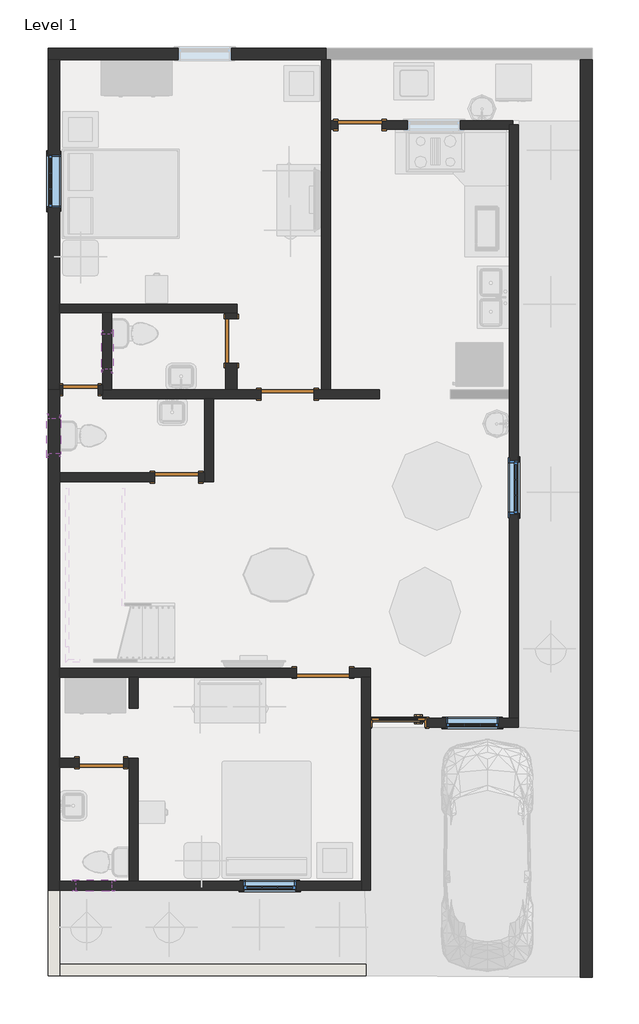
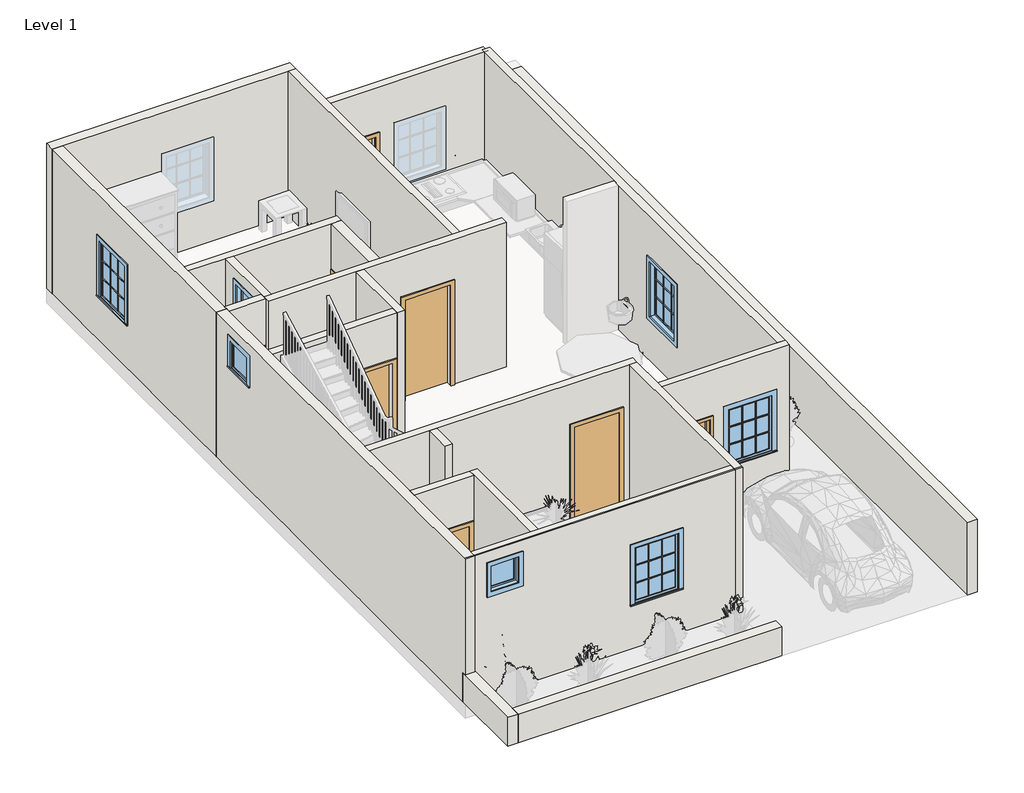
# One storey, part 1 of 3: 23 walls, 8 doors, 7 windows.
"""IFC4 building model written with IfcOpenShell, lengths in millimetres."""

from ifc_helpers import new_model, si_unit, frame, origin, origin_with_axes, place, context, project, spatial, polyline, outline, extrude, faceted_brep, transform, mapped, element, save
from components import door_808aeb8e, door_d7591924, door_fadea3f2, door_255cab33, door_059fdd7e, door_16372e1c, door_686f89d2, window_29c06734, window_5c190c7e, window_3d781103, window_e41d21a6

model = new_model("IFC4")

# Units and contexts
model_context = context("Model", 3, world=origin())
ifc_project = project(units=[si_unit("LENGTHUNIT", "METRE", prefix="MILLI")], contexts=[model_context])

# Site, building, storey
site = spatial("IfcSite", under=ifc_project)
building = spatial("IfcBuilding", under=site)
storey = spatial("IfcBuildingStorey", under=building, Name="Level 1", Elevation=0.0)

# Doors
placement = place(None, origin())
door_shape = door_808aeb8e(model_context)
element("IfcDoor", 1, ObjectType="36\" x 80\"", at=placement, inside=storey, context=model_context, shape_type="MappedRepresentation", body=[
    mapped(door_shape, transform((-8513.5660538, 2790.728629, 0.0), x_axis=(1.0, 0.0, 0.0), y_axis=(0.0, 1.0, 0.0), z_axis=(0.0, 0.0, 1.0))),
])
door_2_shape = door_d7591924(model_context)
element("IfcDoor", 2, ObjectType="Single-Flush : 24\" x 80\"", at=placement, inside=storey, context=model_context, shape_type="MappedRepresentation", body=[
    mapped(door_2_shape, transform((-13974.5660538, 8502.553629, 0.0), x_axis=(1.0, 0.0, 0.0), y_axis=(0.0, 1.0, 0.0), z_axis=(0.0, 0.0, 1.0))),
])
door_3_shape = door_fadea3f2(model_context)
element("IfcDoor", 3, ObjectType="Single-Flush : 30\" x 80\"", at=placement, inside=storey, context=model_context, shape_type="MappedRepresentation", body=[
    mapped(door_3_shape, transform((-11383.7660538, 9340.753629, 0.0), x_axis=(0.0, 1.0, 0.0), y_axis=(-1.0, 0.0, 0.0), z_axis=(0.0, 0.0, 1.0))),
])
door_4_shape = door_255cab33(model_context)
element("IfcDoor", 4, ObjectType="Single-Flush : 30\" x 80\"", at=placement, inside=storey, context=model_context, shape_type="MappedRepresentation", body=[
    mapped(door_4_shape, transform((-9173.9660538, 13049.153629, 0.0), x_axis=(-1.0, 0.0, 0.0), y_axis=(0.0, -1.0, 0.0), z_axis=(0.0, 0.0, 1.0))),
])
element("IfcDoor", 5, ObjectType="Single-Flush : 30\" x 80\"", at=placement, inside=storey, context=model_context, shape_type="MappedRepresentation", body=[
    mapped(door_4_shape, transform((-13618.9660538, 2101.753629, 0.0), x_axis=(1.0, 0.0, 0.0), y_axis=(0.0, 1.0, 0.0), z_axis=(0.0, 0.0, 1.0))),
])
door_5_shape = door_059fdd7e(model_context)
element("IfcDoor", 6, ObjectType="Single-Flush : 30\" x 80\"", at=placement, inside=storey, context=model_context, shape_type="MappedRepresentation", body=[
    mapped(door_5_shape, transform((-12323.5660538, 7003.953629, 0.0), x_axis=(1.0, 0.0, 0.0), y_axis=(0.0, 1.0, 0.0), z_axis=(0.0, 0.0, 1.0))),
])
door_6_shape = door_16372e1c(model_context)
element("IfcDoor", 7, ObjectType="Single-Flush : 36\" x 84\"", at=placement, inside=storey, context=model_context, shape_type="MappedRepresentation", body=[
    mapped(door_6_shape, transform((-10418.5660538, 8426.353629, 0.0), x_axis=(1.0, 0.0, 0.0), y_axis=(0.0, 1.0, 0.0), z_axis=(0.0, 0.0, 1.0))),
])
door_7_shape = door_686f89d2(model_context)
element("IfcDoor", 8, ObjectType="Single-Flush : 36\" x 84\"", at=placement, inside=storey, context=model_context, shape_type="MappedRepresentation", body=[
    mapped(door_7_shape, transform((-9808.9660538, 3651.153629, 0.0), x_axis=(1.0, 0.0, 0.0), y_axis=(0.0, 1.0, 0.0), z_axis=(0.0, 0.0, 1.0))),
])

# Walls
element("IfcWall", 9, ObjectType="Generic - 8\"", at=placement, inside=storey, context=model_context, shape_type="Brep", body=[
    faceted_brep([(-14533.3660538, 14166.753629, 0.0), (-14330.1660538, 14166.753629, 0.0), (-9834.3660538, 14166.753629, 0.0), (-9758.1660538, 14166.753629, 0.0), (-9758.1660538, 14166.753629, 1524.0), (-9681.9660538, 14166.753629, 1524.0), (-9681.9660538, 14166.753629, 3048.0), (-9834.3660538, 14166.753629, 3048.0), (-14330.1660538, 14166.753629, 3048.0), (-14533.3660538, 14166.753629, 3048.0), (-11383.7660538, 14166.753629, 2133.6), (-11383.7660538, 14166.753629, 914.4), (-12298.1660538, 14166.753629, 914.4), (-12298.1660538, 14166.753629, 2133.6), (-14533.3660538, 14369.953629, 0.0), (-14533.3660538, 14369.953629, 3048.0), (-9681.9660538, 14369.953629, 3048.0), (-9681.9660538, 14369.953629, 1524.0), (-9758.1660538, 14369.953629, 1524.0), (-9758.1660538, 14369.953629, 0.0), (-11383.7660538, 14369.953629, 2133.6), (-12298.1660538, 14369.953629, 2133.6), (-12298.1660538, 14369.953629, 914.4), (-11383.7660538, 14369.953629, 914.4)], [[[0, 1, 2, 3, 4, 5, 6, 7, 8, 9], [10, 11, 12, 13]], [[14, 15, 16, 17, 18, 19], [20, 21, 22, 23]], [[3, 2, 1, 0, 14, 19]], [[0, 9, 15, 14]], [[11, 10, 20, 23]], [[12, 11, 23, 22]], [[13, 12, 22, 21]], [[10, 13, 21, 20]], [[4, 3, 19, 18]], [[17, 5, 4, 18]], [[6, 5, 17, 16]], [[9, 8, 7, 6, 16, 15]]]),
])
element("IfcWall", 10, ObjectType="Generic - 8\"", at=placement, inside=storey, context=model_context, shape_type="SweptSolid", body=[
    extrude(outline(polyline([(9823.353629, 0.0), (9721.753629, 0.0), (9721.753629, 2032.0), (8959.753629, 2032.0), (8959.753629, 0.0), (8502.553629, 0.0), (8502.553629, 3048.0), (9823.353629, 3048.0), (9823.353629, 0.0)])), frame((-11485.3660538, 0.0, 0.0), z_axis=(1.0, 0.0, 0.0), x_axis=(0.0, 1.0, 0.0)), (0.0, 0.0, 1.0), 203.2),
])
element("IfcWall", 11, ObjectType="Generic - 8\"", at=placement, inside=storey, context=model_context, shape_type="Brep", body=[
    faceted_brep([(-14330.1660538, 8502.553629, 0.0), (-14330.1660538, 8578.753629, 0.0), (-14330.1660538, 9823.353629, 0.0), (-14330.1660538, 9975.753629, 0.0), (-14330.1660538, 14166.753629, 0.0), (-14330.1660538, 14166.753629, 3048.0), (-14330.1660538, 9975.753629, 3048.0), (-14330.1660538, 9823.353629, 3048.0), (-14330.1660538, 8578.753629, 3048.0), (-14330.1660538, 8502.553629, 3048.0), (-14330.1660538, 12541.153629, 2133.6), (-14330.1660538, 12541.153629, 914.4), (-14330.1660538, 11626.753629, 914.4), (-14330.1660538, 11626.753629, 2133.6), (-14533.3660538, 8502.553629, 0.0), (-14533.3660538, 8502.553629, 3048.0), (-14533.3660538, 14166.753629, 3048.0), (-14533.3660538, 14166.753629, 0.0), (-14533.3660538, 12541.153629, 2133.6), (-14533.3660538, 11626.753629, 2133.6), (-14533.3660538, 11626.753629, 914.4), (-14533.3660538, 12541.153629, 914.4)], [[[0, 1, 2, 3, 4, 5, 6, 7, 8, 9], [10, 11, 12, 13]], [[14, 15, 16, 17], [18, 19, 20, 21]], [[4, 3, 2, 1, 0, 14, 17]], [[0, 9, 15, 14]], [[5, 4, 17, 16]], [[11, 10, 18, 21]], [[12, 11, 21, 20]], [[13, 12, 20, 19]], [[10, 13, 19, 18]], [[9, 8, 7, 6, 5, 16, 15]]]),
])
element("IfcWall", 12, ObjectType="Generic - 8\"", at=placement, inside=storey, context=model_context, shape_type="Brep", body=[
    faceted_brep([(-14330.1660538, -6.446371, 0.0), (-14330.1660538, 69.753629, 0.0), (-14330.1660538, 2025.553629, 0.0), (-14330.1660538, 2177.953629, 0.0), (-14330.1660538, 3574.953629, 0.0), (-14330.1660538, 3727.353629, 0.0), (-14330.1660538, 6927.753629, 0.0), (-14330.1660538, 7080.153629, 0.0), (-14330.1660538, 8426.353629, 0.0), (-14330.1660538, 8502.553629, 0.0), (-14330.1660538, 8502.553629, 3048.0), (-14330.1660538, 8426.353629, 3048.0), (-14330.1660538, 7080.153629, 3048.0), (-14330.1660538, 6927.753629, 3048.0), (-14330.1660538, 3727.353629, 3048.0), (-14330.1660538, 3574.953629, 3048.0), (-14330.1660538, 2177.953629, 3048.0), (-14330.1660538, 2025.553629, 3048.0), (-14330.1660538, 69.753629, 3048.0), (-14330.1660538, -50.896371, 3048.0), (-14330.1660538, -82.646371, 3048.0), (-14330.1660538, -82.646371, 609.6), (-14330.1660538, -6.446371, 609.6), (-14330.1660538, 8019.953629, 2768.6), (-14330.1660538, 8019.953629, 2159.0), (-14330.1660538, 7410.353629, 2159.0), (-14330.1660538, 7410.353629, 2768.6), (-14533.3660538, -6.446371, 0.0), (-14533.3660538, -6.446371, 609.6), (-14533.3660538, -82.646371, 609.6), (-14533.3660538, -82.646371, 3048.0), (-14533.3660538, -50.896371, 3048.0), (-14533.3660538, 8502.553629, 3048.0), (-14533.3660538, 8502.553629, 0.0), (-14533.3660538, 8019.953629, 2768.6), (-14533.3660538, 7410.353629, 2768.6), (-14533.3660538, 7410.353629, 2159.0), (-14533.3660538, 8019.953629, 2159.0)], [[[0, 1, 2, 3, 4, 5, 6, 7, 8, 9, 10, 11, 12, 13, 14, 15, 16, 17, 18, 19, 20, 21, 22], [23, 24, 25, 26]], [[27, 28, 29, 30, 31, 32, 33], [34, 35, 36, 37]], [[9, 8, 7, 6, 5, 4, 3, 2, 1, 0, 27, 33]], [[10, 9, 33, 32]], [[0, 22, 28, 27]], [[21, 29, 28, 22]], [[21, 20, 30, 29]], [[24, 23, 34, 37]], [[25, 24, 37, 36]], [[26, 25, 36, 35]], [[23, 26, 35, 34]], [[20, 19, 31, 30]], [[19, 18, 17, 16, 15, 14, 13, 12, 11, 10, 32, 31]]]),
])
element("IfcWall", 13, ObjectType="Generic - 8\" 2", at=placement, inside=storey, context=model_context, shape_type="SweptSolid", body=[
    extrude(outline(polyline([(-5389.3660538, -1581.246371), (-5389.3660538, 14166.753629), (-5186.1660538, 14166.753629), (-5186.1660538, -1581.246371), (-5389.3660538, -1581.246371)])), origin_with_axes(), (0.0, 0.0, 1.0), 1524.0),
])
element("IfcWall", 14, ObjectType="Generic - 8\" 2", at=placement, inside=storey, context=model_context, shape_type="Brep", body=[
    faceted_brep([(-14330.1660538, -1555.846371, 0.0), (-14330.1660538, -1352.646371, 0.0), (-14330.1660538, -82.646371, 0.0), (-14330.1660538, -6.446371, 0.0), (-14330.1660538, -6.446371, 609.6), (-14330.1660538, -1352.646371, 609.6), (-14330.1660538, -1555.846371, 609.6), (-14533.3660538, -1555.846371, 0.0), (-14533.3660538, -1555.846371, 609.6), (-14533.3660538, -6.446371, 609.6), (-14533.3660538, -6.446371, 0.0)], [[[0, 1, 2, 3, 4, 5, 6]], [[7, 8, 9, 10]], [[3, 2, 1, 0, 7, 10]], [[4, 3, 10, 9]], [[6, 5, 4, 9, 8]], [[0, 6, 8, 7]]]),
])
element("IfcWall", 15, ObjectType="Generic - 8\" 2", at=placement, inside=storey, context=model_context, shape_type="SweptSolid", body=[
    extrude(outline(polyline([(-14330.1660538, -1352.646371), (-9072.3660538, -1352.646371), (-9072.3660538, -1555.846371), (-14330.1660538, -1555.846371), (-14330.1660538, -1352.646371)])), origin_with_axes(), (0.0, 0.0, 1.0), 609.6),
])
element("IfcWall", 16, ObjectType="INNER 6\"", at=placement, inside=storey, context=model_context, shape_type="Brep", body=[
    faceted_brep([(-9834.3660538, 14166.753629, 3048.0), (-9834.3660538, 14166.753629, 0.0), (-9834.3660538, 8502.553629, 0.0), (-9834.3660538, 8502.553629, 3048.0), (-9681.9660538, 14166.753629, 0.0), (-9681.9660538, 14166.753629, 1524.0), (-9681.9660538, 14166.753629, 3048.0), (-9681.9660538, 13125.353629, 3048.0), (-9681.9660538, 12972.953629, 3048.0), (-9681.9660538, 8502.553629, 3048.0), (-9681.9660538, 8502.553629, 0.0), (-9681.9660538, 12972.953629, 0.0), (-9681.9660538, 13125.353629, 0.0), (-9758.1660538, 14166.753629, 0.0)], [[[0, 1, 2, 3]], [[4, 5, 6, 7, 8, 9, 10, 11, 12]], [[2, 1, 13, 4, 12, 11, 10]], [[3, 2, 10, 9]], [[0, 6, 5, 4, 13, 1]], [[0, 3, 9, 8, 7, 6]]]),
])
element("IfcWall", 17, ObjectType="INNER 6\"", at=placement, inside=storey, context=model_context, shape_type="SweptSolid", body=[
    extrude(outline(polyline([(0.0, -9681.9660538), (0.0, -9554.9660538), (2032.0, -9554.9660538), (2032.0, -8792.9660538), (0.0, -8792.9660538), (0.0, -6545.0660538), (3048.0, -6545.0660538), (3048.0, -9681.9660538), (0.0, -9681.9660538)]), holes=[polyline([(2133.6, -7446.7660538), (914.4, -7446.7660538), (914.4, -8361.1660538), (2133.6, -8361.1660538), (2133.6, -7446.7660538)])]), frame((0.0, 12972.953629, 0.0), z_axis=(0.0, 1.0, 0.0), x_axis=(0.0, 0.0, 1.0)), (0.0, 0.0, 1.0), 152.4),
])
element("IfcWall", 18, ObjectType="INNER 6\"", at=placement, inside=storey, context=model_context, shape_type="Brep", body=[
    faceted_brep([(-6456.1660538, 2863.753629, 0.0), (-6456.1660538, 13049.153629, 0.0), (-6456.1660538, 13049.153629, 3048.0), (-6456.1660538, 2863.753629, 3048.0), (-6456.1660538, 6368.953629, 2133.6), (-6456.1660538, 7283.353629, 2133.6), (-6456.1660538, 7283.353629, 914.4), (-6456.1660538, 6368.953629, 914.4), (-6608.5660538, 2863.753629, 0.0), (-6608.5660538, 2863.753629, 3048.0), (-6608.5660538, 8350.153629, 3048.0), (-6608.5660538, 8502.553629, 3048.0), (-6608.5660538, 13049.153629, 3048.0), (-6608.5660538, 13049.153629, 0.0), (-6608.5660538, 8502.553629, 0.0), (-6608.5660538, 8350.153629, 0.0), (-6608.5660538, 6368.953629, 2133.6), (-6608.5660538, 6368.953629, 914.4), (-6608.5660538, 7283.353629, 914.4), (-6608.5660538, 7283.353629, 2133.6)], [[[0, 1, 2, 3], [4, 5, 6, 7]], [[8, 9, 10, 11, 12, 13, 14, 15], [16, 17, 18, 19]], [[1, 0, 8, 15, 14, 13]], [[2, 1, 13, 12]], [[0, 3, 9, 8]], [[17, 16, 4, 7]], [[18, 17, 7, 6]], [[19, 18, 6, 5]], [[16, 19, 5, 4]], [[3, 2, 12, 11, 10, 9]]]),
])
element("IfcWall", 19, ObjectType="INNER 6\"", at=placement, inside=storey, context=model_context, shape_type="Brep", body=[
    faceted_brep([(-14330.1660538, 9823.353629, 0.0), (-13593.5660538, 9823.353629, 0.0), (-13441.1660538, 9823.353629, 0.0), (-11485.3660538, 9823.353629, 0.0), (-11282.1660538, 9823.353629, 0.0), (-11282.1660538, 9823.353629, 3048.0), (-11485.3660538, 9823.353629, 3048.0), (-13441.1660538, 9823.353629, 3048.0), (-13593.5660538, 9823.353629, 3048.0), (-14330.1660538, 9823.353629, 3048.0), (-14330.1660538, 9975.753629, 0.0), (-14330.1660538, 9975.753629, 3048.0), (-11282.1660538, 9975.753629, 3048.0), (-11282.1660538, 9975.753629, 0.0)], [[[0, 1, 2, 3, 4, 5, 6, 7, 8, 9]], [[10, 11, 12, 13]], [[4, 3, 2, 1, 0, 10, 13]], [[0, 9, 11, 10]], [[5, 4, 13, 12]], [[9, 8, 7, 6, 5, 12, 11]]]),
])
element("IfcWall", 20, ObjectType="INNER 6\"", at=placement, inside=storey, context=model_context, shape_type="Brep", body=[
    faceted_brep([(-11840.9660538, 8350.153629, 0.0), (-11840.9660538, 7080.153629, 0.0), (-11840.9660538, 6927.753629, 0.0), (-11840.9660538, 6927.753629, 3048.0), (-11840.9660538, 7080.153629, 3048.0), (-11840.9660538, 8350.153629, 3048.0), (-11688.5660538, 8350.153629, 0.0), (-11688.5660538, 8350.153629, 3048.0), (-11688.5660538, 6927.753629, 3048.0), (-11688.5660538, 6927.753629, 0.0)], [[[0, 1, 2, 3, 4, 5]], [[6, 7, 8, 9]], [[2, 1, 0, 6, 9]], [[0, 5, 7, 6]], [[3, 2, 9, 8]], [[5, 4, 3, 8, 7]]]),
])
element("IfcWall", 21, ObjectType="INNER 6\"", at=placement, inside=storey, context=model_context, shape_type="SweptSolid", body=[
    extrude(outline(polyline([(2032.0, -11942.5660538), (0.0, -11942.5660538), (0.0, -11840.9660538), (3048.0, -11840.9660538), (3048.0, -14330.1660538), (0.0, -14330.1660538), (0.0, -12704.5660538), (2032.0, -12704.5660538), (2032.0, -11942.5660538)])), frame((0.0, 6927.753629, 0.0), z_axis=(0.0, 1.0, 0.0), x_axis=(0.0, 0.0, 1.0)), (0.0, 0.0, 1.0), 152.4),
])
element("IfcWall", 22, ObjectType="INNER 6\"", at=placement, inside=storey, context=model_context, shape_type="Brep", body=[
    faceted_brep([(-9351.7660538, 3574.953629, 2133.6), (-9351.7660538, 3574.953629, 0.0), (-9148.5660538, 3574.953629, 0.0), (-8996.1660538, 3574.953629, 0.0), (-8996.1660538, 3574.953629, 3048.0), (-9148.5660538, 3574.953629, 3048.0), (-12983.9660538, 3574.953629, 3048.0), (-13136.3660538, 3574.953629, 3048.0), (-14330.1660538, 3574.953629, 3048.0), (-14330.1660538, 3574.953629, 0.0), (-13136.3660538, 3574.953629, 0.0), (-12983.9660538, 3574.953629, 0.0), (-10266.1660538, 3574.953629, 0.0), (-10266.1660538, 3574.953629, 2133.6), (-8996.1660538, 3727.353629, 0.0), (-9351.7660538, 3727.353629, 0.0), (-9351.7660538, 3727.353629, 2133.6), (-10266.1660538, 3727.353629, 2133.6), (-10266.1660538, 3727.353629, 0.0), (-14330.1660538, 3727.353629, 0.0), (-14330.1660538, 3727.353629, 3048.0), (-8996.1660538, 3727.353629, 3048.0)], [[[0, 1, 2, 3, 4, 5, 6, 7, 8, 9, 10, 11, 12, 13]], [[14, 15, 16, 17, 18, 19, 20, 21]], [[3, 2, 1, 15, 14]], [[12, 11, 10, 9, 19, 18]], [[9, 8, 20, 19]], [[16, 15, 1, 0]], [[17, 16, 0, 13]], [[18, 17, 13, 12]], [[4, 3, 14, 21]], [[8, 7, 6, 5, 4, 21, 20]]]),
])
element("IfcWall", 23, ObjectType="INNER 6\"", at=placement, inside=storey, context=model_context, shape_type="Brep", body=[
    faceted_brep([(-9148.5660538, 3574.953629, 0.0), (-9148.5660538, 69.753629, 0.0), (-9148.5660538, -82.646371, 0.0), (-9148.5660538, -82.646371, 3048.0), (-9148.5660538, -50.896371, 3048.0), (-9148.5660538, 69.753629, 3048.0), (-9148.5660538, 3574.953629, 3048.0), (-8996.1660538, 3574.953629, 0.0), (-8996.1660538, 3574.953629, 3048.0), (-8996.1660538, 2863.753629, 3048.0), (-8996.1660538, 2711.353629, 3048.0), (-8996.1660538, -50.896371, 3048.0), (-8996.1660538, -82.646371, 3048.0), (-8996.1660538, -82.646371, 0.0)], [[[0, 1, 2, 3, 4, 5, 6]], [[7, 8, 9, 10, 11, 12, 13]], [[2, 1, 0, 7, 13]], [[0, 6, 8, 7]], [[3, 2, 13, 12]], [[4, 3, 12, 11]], [[6, 5, 4, 11, 10, 9, 8]]]),
])
element("IfcWall", 24, ObjectType="INNER 6\"", at=placement, inside=storey, context=model_context, shape_type="Brep", body=[
    faceted_brep([(-9148.5660538, 69.753629, 0.0), (-12983.9660538, 69.753629, 0.0), (-13136.3660538, 69.753629, 0.0), (-14330.1660538, 69.753629, 0.0), (-14330.1660538, 69.753629, 3048.0), (-13136.3660538, 69.753629, 3048.0), (-12983.9660538, 69.753629, 3048.0), (-9148.5660538, 69.753629, 3048.0), (-11180.5660538, 69.753629, 2133.6), (-11180.5660538, 69.753629, 914.4), (-10266.1660538, 69.753629, 914.4), (-10266.1660538, 69.753629, 2133.6), (-13441.1660538, 69.753629, 2768.6), (-14050.7660538, 69.753629, 2768.6), (-14050.7660538, 69.753629, 2159.0), (-13441.1660538, 69.753629, 2159.0), (-9148.5660538, -82.646371, 0.0), (-9148.5660538, -82.646371, 3048.0), (-14330.1660538, -82.646371, 3048.0), (-14330.1660538, -82.646371, 609.6), (-14330.1660538, -82.646371, 0.0), (-11180.5660538, -82.646371, 2133.6), (-10266.1660538, -82.646371, 2133.6), (-10266.1660538, -82.646371, 914.4), (-11180.5660538, -82.646371, 914.4), (-13441.1660538, -82.646371, 2768.6), (-13441.1660538, -82.646371, 2159.0), (-14050.7660538, -82.646371, 2159.0), (-14050.7660538, -82.646371, 2768.6), (-14330.1660538, -6.446371, 0.0), (-9148.5660538, -50.896371, 3048.0), (-14330.1660538, -50.896371, 3048.0)], [[[0, 1, 2, 3, 4, 5, 6, 7], [8, 9, 10, 11], [12, 13, 14, 15]], [[16, 17, 18, 19, 20], [21, 22, 23, 24], [25, 26, 27, 28]], [[3, 2, 1, 0, 16, 20, 29]], [[0, 7, 30, 17, 16]], [[3, 29, 20, 19, 18, 31, 4]], [[9, 8, 21, 24]], [[10, 9, 24, 23]], [[11, 10, 23, 22]], [[8, 11, 22, 21]], [[26, 25, 12, 15]], [[27, 26, 15, 14]], [[28, 27, 14, 13]], [[25, 28, 13, 12]], [[31, 18, 17, 30]], [[7, 6, 5, 4, 31, 30]]]),
])
element("IfcWall", 25, ObjectType="INNER 6\"", at=placement, inside=storey, context=model_context, shape_type="Brep", body=[
    faceted_brep([(-13593.5660538, 9823.353629, 0.0), (-13593.5660538, 8578.753629, 0.0), (-13593.5660538, 8502.553629, 0.0), (-13593.5660538, 8502.553629, 3048.0), (-13593.5660538, 8578.753629, 3048.0), (-13593.5660538, 9823.353629, 3048.0), (-13593.5660538, 8858.153629, 2768.6), (-13593.5660538, 8858.153629, 2159.0), (-13593.5660538, 9467.753629, 2159.0), (-13593.5660538, 9467.753629, 2768.6), (-13441.1660538, 9823.353629, 0.0), (-13441.1660538, 9823.353629, 3048.0), (-13441.1660538, 8502.553629, 3048.0), (-13441.1660538, 8502.553629, 0.0), (-13441.1660538, 8858.153629, 2768.6), (-13441.1660538, 9467.753629, 2768.6), (-13441.1660538, 9467.753629, 2159.0), (-13441.1660538, 8858.153629, 2159.0)], [[[0, 1, 2, 3, 4, 5], [6, 7, 8, 9]], [[10, 11, 12, 13], [14, 15, 16, 17]], [[2, 1, 0, 10, 13]], [[0, 5, 11, 10]], [[7, 6, 14, 17]], [[8, 7, 17, 16]], [[9, 8, 16, 15]], [[6, 9, 15, 14]], [[3, 2, 13, 12]], [[5, 4, 3, 12, 11]]]),
])
element("IfcWall", 26, ObjectType="INNER 6\"", at=placement, inside=storey, context=model_context, shape_type="Brep", body=[
    faceted_brep([(-8843.7660538, 8502.553629, 0.0), (-9681.9660538, 8502.553629, 0.0), (-9834.3660538, 8502.553629, 0.0), (-9961.3660538, 8502.553629, 0.0), (-9961.3660538, 8502.553629, 2133.6), (-10875.7660538, 8502.553629, 2133.6), (-10875.7660538, 8502.553629, 0.0), (-11282.1660538, 8502.553629, 0.0), (-11485.3660538, 8502.553629, 0.0), (-13441.1660538, 8502.553629, 0.0), (-13593.5660538, 8502.553629, 0.0), (-13593.5660538, 8502.553629, 3048.0), (-13441.1660538, 8502.553629, 3048.0), (-11485.3660538, 8502.553629, 3048.0), (-11282.1660538, 8502.553629, 3048.0), (-9834.3660538, 8502.553629, 3048.0), (-9681.9660538, 8502.553629, 3048.0), (-8843.7660538, 8502.553629, 3048.0), (-9961.3660538, 8350.153629, 2133.6), (-9961.3660538, 8350.153629, 0.0), (-8843.7660538, 8350.153629, 0.0), (-8843.7660538, 8350.153629, 3048.0), (-11688.5660538, 8350.153629, 3048.0), (-11840.9660538, 8350.153629, 3048.0), (-13593.5660538, 8350.153629, 3048.0), (-13593.5660538, 8350.153629, 0.0), (-11840.9660538, 8350.153629, 0.0), (-11688.5660538, 8350.153629, 0.0), (-10875.7660538, 8350.153629, 0.0), (-10875.7660538, 8350.153629, 2133.6), (-13593.5660538, 8426.353629, 0.0), (-13593.5660538, 8426.353629, 3048.0)], [[[0, 1, 2, 3, 4, 5, 6, 7, 8, 9, 10, 11, 12, 13, 14, 15, 16, 17]], [[18, 19, 20, 21, 22, 23, 24, 25, 26, 27, 28, 29]], [[20, 19, 3, 2, 1, 0]], [[28, 27, 26, 25, 30, 10, 9, 8, 7, 6]], [[0, 17, 21, 20]], [[6, 5, 29, 28]], [[5, 4, 18, 29]], [[4, 3, 19, 18]], [[11, 10, 30, 25, 24, 31]], [[17, 16, 15, 14, 13, 12, 11, 31, 24, 23, 22, 21]]]),
])
element("IfcWall", 27, ObjectType="INNER 6\"", at=placement, inside=storey, context=model_context, shape_type="SweptSolid", body=[
    extrude(outline(polyline([(2032.0, -13237.9660538), (0.0, -13237.9660538), (0.0, -13136.3660538), (3048.0, -13136.3660538), (3048.0, -14330.1660538), (0.0, -14330.1660538), (0.0, -13999.9660538), (2032.0, -13999.9660538), (2032.0, -13237.9660538)])), frame((0.0, 2025.553629, 0.0), z_axis=(0.0, 1.0, 0.0), x_axis=(0.0, 0.0, 1.0)), (0.0, 0.0, 1.0), 152.4),
])
element("IfcWall", 28, ObjectType="INNER 6\"", at=placement, inside=storey, context=model_context, shape_type="Brep", body=[
    faceted_brep([(-12983.9660538, 69.753629, 0.0), (-12983.9660538, 2177.953629, 0.0), (-12983.9660538, 2177.953629, 3048.0), (-12983.9660538, 69.753629, 3048.0), (-13136.3660538, 69.753629, 0.0), (-13136.3660538, 69.753629, 3048.0), (-13136.3660538, 2025.553629, 3048.0), (-13136.3660538, 2177.953629, 3048.0), (-13136.3660538, 2177.953629, 0.0), (-13136.3660538, 2025.553629, 0.0)], [[[0, 1, 2, 3]], [[4, 5, 6, 7, 8, 9]], [[1, 0, 4, 9, 8]], [[0, 3, 5, 4]], [[2, 1, 8, 7]], [[3, 2, 7, 6, 5]]]),
])
element("IfcWall", 29, ObjectType="INNER 6\"", at=placement, inside=storey, context=model_context, shape_type="SweptSolid", body=[
    extrude(outline(polyline([(-12983.9660538, 3574.953629), (-12983.9660538, 3041.553629), (-13136.3660538, 3041.553629), (-13136.3660538, 3574.953629), (-12983.9660538, 3574.953629)])), origin_with_axes(), (0.0, 0.0, 1.0), 3048.0),
])
element("IfcWall", 30, ObjectType="INNER 6\"", at=placement, inside=storey, context=model_context, shape_type="Brep", body=[
    faceted_brep([(-6456.1660538, 2711.353629, 0.0), (-6456.1660538, 2711.353629, 3048.0), (-8996.1660538, 2711.353629, 3048.0), (-8996.1660538, 2711.353629, 2057.4), (-8030.9660538, 2711.353629, 2057.4), (-8030.9660538, 2711.353629, 0.0), (-7700.7660538, 2711.353629, 2133.6), (-6786.3660538, 2711.353629, 2133.6), (-6786.3660538, 2711.353629, 914.4), (-7700.7660538, 2711.353629, 914.4), (-6456.1660538, 2863.753629, 3048.0), (-6456.1660538, 2863.753629, 0.0), (-6608.5660538, 2863.753629, 0.0), (-8030.9660538, 2863.753629, 0.0), (-8030.9660538, 2863.753629, 2057.4), (-8996.1660538, 2863.753629, 2057.4), (-8996.1660538, 2863.753629, 3048.0), (-6608.5660538, 2863.753629, 3048.0), (-7700.7660538, 2863.753629, 2133.6), (-7700.7660538, 2863.753629, 914.4), (-6786.3660538, 2863.753629, 914.4), (-6786.3660538, 2863.753629, 2133.6)], [[[0, 1, 2, 3, 4, 5], [6, 7, 8, 9]], [[10, 11, 12, 13, 14, 15, 16, 17], [18, 19, 20, 21]], [[11, 0, 5, 13, 12]], [[2, 16, 15, 3]], [[1, 0, 11, 10]], [[4, 14, 13, 5]], [[14, 4, 3, 15]], [[19, 18, 6, 9]], [[20, 19, 9, 8]], [[21, 20, 8, 7]], [[18, 21, 7, 6]], [[2, 1, 10, 17, 16]]]),
])
element("IfcWall", 31, ObjectType="INNER 6\"", at=placement, inside=storey, context=model_context, shape_type="Brep", body=[
    faceted_brep([(-13593.5660538, 8578.753629, 3048.0), (-13593.5660538, 8578.753629, 0.0), (-13669.7660538, 8578.753629, 0.0), (-13669.7660538, 8578.753629, 2032.0), (-14279.3660538, 8578.753629, 2032.0), (-14279.3660538, 8578.753629, 0.0), (-14330.1660538, 8578.753629, 0.0), (-14330.1660538, 8578.753629, 3048.0), (-13593.5660538, 8426.353629, 0.0), (-13593.5660538, 8426.353629, 3048.0), (-14330.1660538, 8426.353629, 3048.0), (-14330.1660538, 8426.353629, 0.0), (-14279.3660538, 8426.353629, 0.0), (-14279.3660538, 8426.353629, 2032.0), (-13669.7660538, 8426.353629, 2032.0), (-13669.7660538, 8426.353629, 0.0), (-13593.5660538, 8502.553629, 0.0), (-14330.1660538, 8502.553629, 0.0), (-13593.5660538, 8502.553629, 3048.0), (-14330.1660538, 8502.553629, 3048.0)], [[[0, 1, 2, 3, 4, 5, 6, 7]], [[8, 9, 10, 11, 12, 13, 14, 15]], [[1, 16, 8, 15, 2]], [[11, 17, 6, 5, 12]], [[1, 0, 18, 9, 8, 16]], [[7, 6, 17, 11, 10, 19]], [[14, 3, 2, 15]], [[3, 14, 13, 4]], [[4, 13, 12, 5]], [[0, 7, 19, 10, 9, 18]]]),
])

# Windows
window_shape = window_29c06734(model_context)
element("IfcWindow", 32, ObjectType="Casement 3x3 with Trim : 36\" x 48\"", at=placement, inside=storey, context=model_context, shape_type="MappedRepresentation", body=[
    mapped(window_shape, transform((-14431.7660538, 12083.953629, 0.0), x_axis=(0.0, 1.0, 0.0), y_axis=(-1.0, 0.0, 0.0), z_axis=(0.0, 0.0, 1.0))),
])
window_2_shape = window_5c190c7e(model_context)
element("IfcWindow", 33, ObjectType="Casement 3x3 with Trim : 36\" x 48\"", at=placement, inside=storey, context=model_context, shape_type="MappedRepresentation", body=[
    mapped(window_2_shape, transform((-7243.5660538, 2787.553629, 0.0), x_axis=(-1.0, 0.0, 0.0), y_axis=(0.0, -1.0, 0.0), z_axis=(0.0, 0.0, 1.0))),
])
element("IfcWindow", 34, ObjectType="Casement 3x3 with Trim : 36\" x 48\"", at=placement, inside=storey, context=model_context, shape_type="MappedRepresentation", body=[
    mapped(window_2_shape, transform((-6532.3660538, 6826.153629, 0.0), x_axis=(0.0, -1.0, 0.0), y_axis=(1.0, 0.0, 0.0), z_axis=(0.0, 0.0, 1.0))),
])
element("IfcWindow", 35, ObjectType="Casement 3x3 with Trim : 36\" x 48\"", at=placement, inside=storey, context=model_context, shape_type="MappedRepresentation", body=[
    mapped(window_2_shape, transform((-10723.3660538, -6.446371, 0.0), x_axis=(-1.0, 0.0, 0.0), y_axis=(0.0, -1.0, 0.0), z_axis=(0.0, 0.0, 1.0))),
])
window_3_shape = window_3d781103(model_context)
element("IfcWindow", 36, ObjectType="Transom with Trim : 24\" x 24\"", at=placement, inside=storey, context=model_context, shape_type="MappedRepresentation", body=[
    mapped(window_3_shape, transform((-13707.8660538, -6.446371, 0.0), x_axis=(1.0, 0.0, 0.0), y_axis=(0.0, 1.0, 0.0), z_axis=(0.0, 0.0, 1.0))),
])
element("IfcWindow", 37, ObjectType="Transom with Trim : 24\" x 24\"", at=placement, inside=storey, context=model_context, shape_type="MappedRepresentation", body=[
    mapped(window_3_shape, transform((-13517.3660538, 9124.853629, 0.0), x_axis=(0.0, -1.0, 0.0), y_axis=(1.0, 0.0, 0.0), z_axis=(0.0, 0.0, 1.0))),
])
window_4_shape = window_e41d21a6(model_context)
element("IfcWindow", 38, ObjectType="Transom with Trim : 24\" x 24\"", at=placement, inside=storey, context=model_context, shape_type="MappedRepresentation", body=[
    mapped(window_4_shape, transform((-14431.7660538, 7753.253629, 0.0), x_axis=(0.0, 1.0, 0.0), y_axis=(-1.0, 0.0, 0.0), z_axis=(0.0, 0.0, 1.0))),
])

save(model, "model.ifc")

# Revit data of these elements
# Type "36\" x 80\""
#   Type Mark = "8"
#   Assembly Code = "B2030100"
#   Analytic Construction = "French door, wood frame with single glass"
#   Threshold Offset [instance default] = 0' - 0 1/2"
#   Thickness = 0' - 1 3/8"
#   Thermal Resistance (R) = 1.0696 (h·ft²·°F)/BTU
#   Swing Angle [instance default] = 90.00°
#   Stiles = 0' - 4 3/4"
#   Rough Width = 3' - 2"
#   Rough Height = 6' - 9"
#   Radius = 1' - 8.05625"
#   Lock Rail = 0' - 7 1/8"
#   Height = 6' - 8"
#   Width = 3' - 0"
#   Heat Transfer Coefficient (U) = 0.9350 BTU/(h·ft²·°F)
#   Door Offset [instance default] = 0' - 0"
#   Bottom Rail = 0' - 9 1/2"
#   Threshold [instance default] = yes
#   Function = 1
#   Exterior Trim [instance default] = yes
#   Trim Material = Cherry
#   Threshold Material = Cherry
#   Panel Material = Cherry
#   Glazing = Glass
#   Frame Material = Cherry
#   Door Handle Material = Aluminum
#   Visual Light Transmittance = 0
#   Solar Heat Gain Coefficient = 0
#   Wall Closure = (empty or 0)
#   Construction Type = (empty or 0)
# Type "Single-Flush : 24\" x 80\""
#   Type Mark = "9"
#   Construction Type Id = "MDOOR"
#   Assembly Code = "C1020"
#   Analytic Construction = "Metal"
#   Thickness = 0' - 2"
#   Heat Transfer Coefficient (U) = 0.651978 BTU/(h·ft²·°F)
#   Height = 6' - 8"
#   Trim Projection Ext = 0' - 1"
#   Trim Projection Int = 0' - 1"
#   Trim Width = 0' - 2"
#   Width = 2' - 0"
#   Define Thermal Properties by = 1
#   Door Material = Door - Panel
#   Frame Material = Door - Frame
#   Visual Light Transmittance = 0
#   Solar Heat Gain Coefficient = 0
#   Function = (empty or 0)
#   Wall Closure = (empty or 0)
# Type "Single-Flush : 30\" x 80\""
#   Type Mark = "5"
#   Construction Type Id = "MDOOR"
#   Assembly Code = "C1020"
#   Analytic Construction = "Metal"
#   Thickness = 0' - 2"
#   Heat Transfer Coefficient (U) = 0.651978 BTU/(h·ft²·°F)
#   Height = 6' - 8"
#   Trim Projection Ext = 0' - 1"
#   Trim Projection Int = 0' - 1"
#   Trim Width = 0' - 3"
#   Width = 2' - 6"
#   Define Thermal Properties by = 1
#   Door Material = Door - Panel
#   Frame Material = Door - Frame
#   Visual Light Transmittance = 0
#   Solar Heat Gain Coefficient = 0
#   Function = (empty or 0)
#   Wall Closure = (empty or 0)
# Type "Single-Flush : 36\" x 84\""
#   Type Mark = "1"
#   Construction Type Id = "MDOOR"
#   Assembly Code = "C1020"
#   Analytic Construction = "Metal"
#   Thickness = 0' - 2"
#   Heat Transfer Coefficient (U) = 0.651978 BTU/(h·ft²·°F)
#   Height = 7' - 0"
#   Trim Projection Ext = 0' - 1"
#   Trim Projection Int = 0' - 1"
#   Trim Width = 0' - 3"
#   Width = 3' - 0"
#   Define Thermal Properties by = 1
#   Door Material = Door - Panel
#   Frame Material = Door - Frame
#   Visual Light Transmittance = 0
#   Solar Heat Gain Coefficient = 0
#   Function = (empty or 0)
#   Wall Closure = (empty or 0)
# Type "Generic - 8\""
#   Assembly Code = "B2010"
#   Layers, outside or top first: 0' - 8" "Brick, Common" (function 1)
# Type "Generic - 8\" 2"
#   Assembly Code = "B2010"
#   Layers, outside or top first: 0' - 8" "Birch" (function 1)
# Type "INNER 6\""
#   Assembly Code = "B2010"
#   Layers, outside or top first: 0' - 6" "Brick, Common" (function 1)
# Type "Casement 3x3 with Trim : 36\" x 48\""
#   Type Mark = "10"
#   Construction Type Id = "GSP4R"
#   Assembly Code = "B2020100"
#   Analytic Construction = "1/8 in Pilkington single glazing"
#   Visual Light Transmittance = 0.9
#   Solar Heat Gain Coefficient = 0.78
#   Heat Transfer Coefficient (U) = 0.6496 BTU/(h·ft²·°F)
#   Height = 4' - 0"
#   Default Sill Height = 3' - 0"
#   Trim Projection - Ext. = 0' - 0 1/2"
#   Trim Projection - Int. = 0' - 0 3/4"
#   Trim Width - Exterior = 0' - 3 1/2"
#   Trim Width - Interior = 0' - 3 1/2"
#   Width = 3' - 0"
#   Window Inset = 0' - 0 3/4"
#   Define Thermal Properties by = 1
#   Glass Pane Material = Glass
#   Sash Material = Sash
#   Trim Exterior Material = Trim
#   Trim Interior Material = Trim
#   Wall Closure = (empty or 0)
# Type "Transom with Trim : 24\" x 24\""
#   Type Mark = "13"
#   Construction Type Id = "GSP4R"
#   Assembly Code = "B2020100"
#   Analytic Construction = "1/8 in Pilkington single glazing"
#   Visual Light Transmittance = 0.9
#   Solar Heat Gain Coefficient = 0.78
#   Heat Transfer Coefficient (U) = 0.6496 BTU/(h·ft²·°F)
#   Height = 2' - 0"
#   Default Sill Height = 7' - 1"
#   Trim Projection - Ext. = 0' - 0 1/2"
#   Trim Projection - Int. = 0' - 0 3/4"
#   Trim Width - Exterior = 0' - 3 1/2"
#   Trim Width - Interior = 0' - 3 1/2"
#   Width = 2' - 0"
#   Window Inset = 0' - 0 3/4"
#   Define Thermal Properties by = 1
#   Glass Pane Material = Glass
#   Sash Material = Sash
#   Trim Exterior Material = Trim
#   Trim Interior Material = Trim
#   Wall Closure = (empty or 0)
# Element 1 (IfcDoor, "36\" x 80\"")
#   Threshold Offset = 0' - 0 1/2"
#   Swing Angle = 90.00°
#   Door Offset = 0' - 0"
#   Threshold = yes
#   Exterior Trim = yes
#   Phase Created = New Construction
#   Materials on its faces: "Cherry", "Aluminum", "Glass"
# Element 2 (IfcDoor, "Single-Flush : 24\" x 80\"")
#   Phase Created = New Construction
#   Materials on its faces: "Door - Frame", "Door - Panel"
# Elements 3, 4, 5, 6 (IfcDoor, "Single-Flush : 30\" x 80\"")
#   Phase Created = New Construction
#   Materials on its faces: "Door - Frame", "Door - Panel"
# Elements 7, 8 (IfcDoor, "Single-Flush : 36\" x 84\"")
#   Phase Created = New Construction
#   Materials on its faces: "Door - Frame", "Door - Panel"
# Elements 9, 10, 11, 12 (IfcWall, "Generic - 8\"")
#   Top Offset = 0' - 0"
#   Base Offset = 0' - 0"
#   Unconnected Height = 10' - 0"
#   wall height = 10' - 0"
#   Phase Created = New Construction
#   Base Constraint = Level 1
#   Materials on its faces: "Brick, Common"
# Element 13 (IfcWall, "Generic - 8\" 2")
#   Top Offset = 0' - 0"
#   Base Offset = 0' - 0"
#   Unconnected Height = 5' - 0"
#   wall height = 5' - 0"
#   Phase Created = New Construction
#   Base Constraint = Level 1
#   Materials on its faces: "Birch"
# Elements 14, 15 (IfcWall, "Generic - 8\" 2")
#   Top Offset = 0' - 0"
#   Base Offset = 0' - 0"
#   Unconnected Height = 2' - 0"
#   wall height = 2' - 0"
#   Phase Created = New Construction
#   Base Constraint = Level 1
#   Materials on its faces: "Birch"
# Elements 16, 17, 18, 19, 20, 21, 22, 23, 24, 25, 26, 27, 28, 29, 30, 31 (IfcWall, "INNER 6\"")
#   Top Offset = 0' - 0"
#   Base Offset = 0' - 0"
#   Unconnected Height = 10' - 0"
#   wall height = 10' - 0"
#   Phase Created = New Construction
#   Base Constraint = Level 1
#   Materials on its faces: "Brick, Common"
# Element 32 (IfcWindow, "Casement 3x3 with Trim : 36\" x 48\"")
#   Mark = "3"
#   Phase Created = New Construction
#   Materials on its faces: "Sash", "Glass", "Trim"
# Element 33 (IfcWindow, "Casement 3x3 with Trim : 36\" x 48\"")
#   Mark = "5"
#   Phase Created = New Construction
#   Materials on its faces: "Sash", "Glass", "Trim"
# Element 34 (IfcWindow, "Casement 3x3 with Trim : 36\" x 48\"")
#   Mark = "6"
#   Phase Created = New Construction
#   Materials on its faces: "Sash", "Glass", "Trim"
# Element 35 (IfcWindow, "Casement 3x3 with Trim : 36\" x 48\"")
#   Mark = "7"
#   Phase Created = New Construction
#   Materials on its faces: "Sash", "Glass", "Trim"
# Element 36 (IfcWindow, "Transom with Trim : 24\" x 24\"")
#   Mark = "8"
#   Phase Created = New Construction
#   Materials on its faces: "Sash", "Trim", "Glass"
# Element 37 (IfcWindow, "Transom with Trim : 24\" x 24\"")
#   Mark = "10"
#   Phase Created = New Construction
#   Materials on its faces: "Sash", "Trim", "Glass"
# Element 38 (IfcWindow, "Transom with Trim : 24\" x 24\"")
#   Mark = "9"
#   Phase Created = New Construction
#   Materials on its faces: "Sash", "Trim", "Glass"
# Materials
#   "Cherry": class "Wood", colour RGB 226 177 128, transparency 0, Description = "Prunus Serotina", Cost = 0
#   "Glass": class "Glass", colour RGB 0 128 192, transparency 0.75, Description = "Soda Lime Glass", Cost = 0
#   "Aluminum": class "Metal", colour RGB 247 247 247, transparency 0, Description = "Aluminum 6061", Cost = 0
#   "Door - Panel": class "Wood", colour RGB 210 159 95, transparency 0
#   "Door - Frame": colour RGB 118 70 51, transparency 0
#   "Brick, Common": class "Masonry", colour RGB 170 98 104, transparency 0, Description = "Common brick", Cost = 0
#   "Birch": class "Wood", colour RGB 224 178 126, transparency 0, Description = "Betula Alleghaniensis", Cost = 0
#   "Sash": class "Wood", colour RGB 224 178 126, transparency 0
#   "Trim": class "Wood", colour RGB 224 178 126, transparency 0
# Room at (-7028.879, 577.399) mm, phase "New Construction", upper level "Level 1", upper offset 10' - 0", lower offset 0' - 0"
#   Number = "11"
#   Name = "PARKING"
# Room at (-11783.419, -905.391) mm, phase "New Construction", upper level "Level 1", upper offset 10' - 0", lower offset 0' - 0"
#   Number = "12"
#   Name = "GARDEN"
# Room at (-12117.142, 11915.456) mm, phase "New Construction", upper level "Level 1", upper offset 10' - 0", lower offset 0' - 0"
#   Number = "1"
#   Name = "BEDROOM-1"
# Room at (-12293.654, 8893.886) mm, phase "New Construction", upper level "Level 1", upper offset 10' - 0", lower offset 0' - 0"
#   Number = "2"
#   Name = "TOILET"
# Room at (-13234.709, 7631.73) mm, phase "New Construction", upper level "Level 1", upper offset 10' - 0", lower offset 0' - 0"
#   Number = "3"
# Room at (-13688.419, 2550.716) mm, phase "New Construction", upper level "Level 1", upper offset 10' - 0", lower offset 0' - 0"
#   Number = "4"
# Room at (-13688.419, 799.081) mm, phase "New Construction", upper level "Level 1", upper offset 10' - 0", lower offset 0' - 0"
#   Number = "5"
#   Name = "TOILET"
# Room at (-11367.537, 1517.471) mm, phase "New Construction", upper level "Level 1", upper offset 10' - 0", lower offset 0' - 0"
#   Number = "6"
#   Name = "BEDROOM-2"
# Room at (-8372.987, 10156.041) mm, phase "New Construction", upper level "Level 1", upper offset 10' - 0", lower offset 0' - 0"
#   Number = "7"
#   Name = "KITCHEN"
# Room at (-7431.78, 13489.331) mm, phase "New Construction", upper level "Level 1", upper offset 10' - 0", lower offset 0' - 0"
#   Number = "8"
#   Name = "WASH"
# Room at (-12989.125, 5281.708) mm, phase "New Construction", upper level "Level 1", upper offset 10' - 0", lower offset 0' - 0"
#   Number = "9"
#   Name = "STAIRS"
# Room at (-9074.153, 5958.081) mm, phase "New Construction", upper level "Level 1", upper offset 10' - 0", lower offset 0' - 0"
#   Number = "10"
#   Name = "LIVING/DINING"
